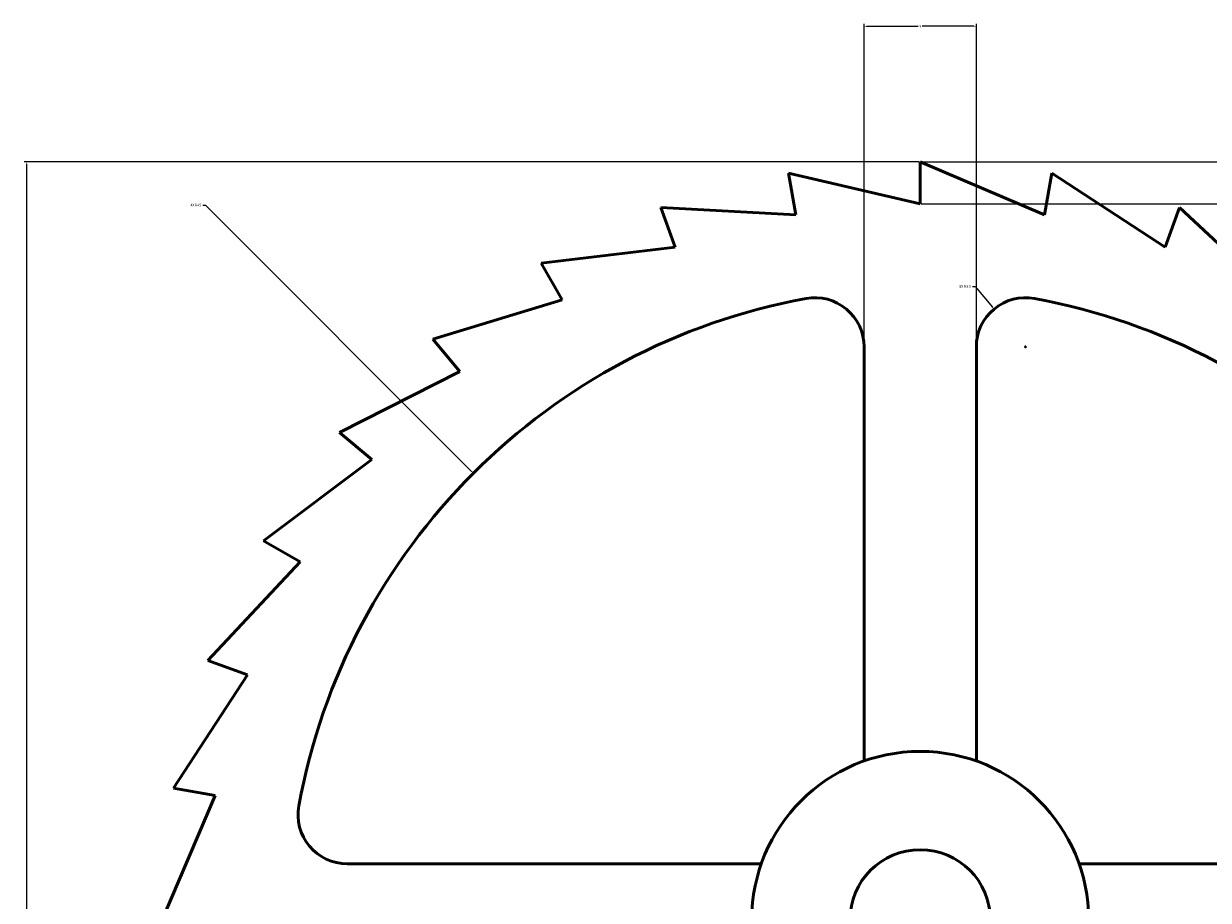
# Model space of a CAD drawing. Units: millimetres. Extents: x 3287 to 3415, y 1573 to 1701.
# Tile 2 of 3: x 3287 to 3371, y 1639 to 1701. Entities that reach past the tile are written whole.
import ezdxf

# ---------------------------------------------------------------- set-up
doc = ezdxf.new("R2010")
doc.units = ezdxf.units.MM
doc.layers.add('M-DIMS', color=2, linetype='Continuous', lineweight=18)
doc.layers.add('M-OUTL', color=7, linetype='Continuous', lineweight=50)
doc.styles.get("Standard").update_dxf_attribs({"font": 'arial.ttf'})
doc.dimstyles.get("Standard").update_dxf_attribs({"dimtxt": 0.18, "dimasz": 0.18, "dimexe": 0.18, "dimexo": 0.0625, "dimgap": 0.09, "dimtad": 0, "dimtih": 1, "dimtoh": 1, "dimdec": 4, "dimzin": 0, "dimdsep": 46, "dimtxsty": 'Standard', "dimcen": 0.09, "dimadec": 0, "dimazin": 0, "dimtfac": 1, "dimtdec": 4, "dimtofl": 0, "dimtmove": 0, "dimatfit": 3, "dimfxl": 1, "dimtolj": 1, "dimtzin": 0, "dimarcsym": 0})

# ---------------------------------------------------------------- blocks, each defined once
blk = doc.blocks.new('RATCHET-TOOTH-10DEG')
for p, q in [((0, 8.856), (2.954, 9.377)), ((2.954, 9.377), (0.775, 0))]:
    blk.add_line(p, q)
blk = doc.blocks.new('WHEEL-SPOKE-OPENING')
for points in [[(40.317, 7.314), (40.317, 36.817)], [(3.5, 0), (33.003, 0)]]:
    blk.add_lwpolyline(points)
for centre, radius, start, end in [((44.317, -4), 45, 100.41187, 169.58813), ((36.817, 36.817), 3.5, 0, 100.41187), ((3.5, 3.5), 3.5, 169.58813, 270)]:
    blk.add_arc(centre, radius, start, end)
blk = doc.blocks.new('*D4')
at = {"layer": 'Defpoints', "color": 0, "transparency": 16777216}
for p in [(3287.322, 1691.286), (3350.972, 1691.286), (3350.972, 1583.286)]:
    blk.add_point(p, dxfattribs=at)
at = {"layer": 'M-DIMS', "color": 0, "lineweight": -2, "transparency": 16777216}
for p, q in [((3350.909, 1691.286), (3287.142, 1691.286)), ((3287.322, 1691.106), (3287.322, 1637.468)), ((3287.322, 1583.466), (3287.322, 1637.104)), ((3350.909, 1583.286), (3287.142, 1583.286))]:
    blk.add_line(p, q, dxfattribs=at)
at = {"layer": 'M-DIMS', "color": 0, "transparency": 16777216}
for points in [[(3287.292, 1691.106), (3287.352, 1691.106), (3287.322, 1691.286)], [(3287.292, 1583.466), (3287.352, 1583.466), (3287.322, 1583.286)]]:
    blk.add_solid(points, dxfattribs=at)
at = {"layer": 'M-DIMS', "color": 0, "transparency": 16777216, "insert": (3287.322, 1637.286), "char_height": 0.18, "attachment_point": 5}
blk.add_mtext('\\A1;108', dxfattribs=at)
blk = doc.blocks.new('*D5')
at = {"layer": 'Defpoints', "color": 0, "transparency": 16777216}
for p in [(3350.972, 1691.286), (3350.972, 1688.286), (3414.622, 1688.286)]:
    blk.add_point(p, dxfattribs=at)
at = {"layer": 'M-DIMS', "color": 0, "lineweight": -2, "transparency": 16777216}
for p, q in [((3351.034, 1691.286), (3414.802, 1691.286)), ((3414.622, 1691.106), (3414.622, 1689.968)), ((3414.622, 1688.466), (3414.622, 1689.604)), ((3351.034, 1688.286), (3414.802, 1688.286))]:
    blk.add_line(p, q, dxfattribs=at)
at = {"layer": 'M-DIMS', "color": 0, "transparency": 16777216}
for points in [[(3414.592, 1691.106), (3414.652, 1691.106), (3414.622, 1691.286)], [(3414.592, 1688.466), (3414.652, 1688.466), (3414.622, 1688.286)]]:
    blk.add_solid(points, dxfattribs=at)
at = {"layer": 'M-DIMS', "color": 0, "transparency": 16777216, "insert": (3414.622, 1689.786), "char_height": 0.18, "attachment_point": 5}
blk.add_mtext('\\A1;3', dxfattribs=at)
blk = doc.blocks.new('*D6')
at = {"layer": 'Defpoints', "color": 0, "transparency": 16777216}
for p in [(3354.972, 1700.936), (3346.972, 1678.103), (3354.972, 1678.103)]:
    blk.add_point(p, dxfattribs=at)
at = {"layer": 'M-DIMS', "color": 0, "lineweight": -2, "transparency": 16777216}
for p, q in [((3346.972, 1678.165), (3346.972, 1701.116)), ((3354.972, 1678.165), (3354.972, 1701.116)), ((3347.152, 1700.936), (3350.822, 1700.936)), ((3354.792, 1700.936), (3351.121, 1700.936))]:
    blk.add_line(p, q, dxfattribs=at)
at = {"layer": 'M-DIMS', "color": 0, "transparency": 16777216}
for points in [[(3347.152, 1700.966), (3347.152, 1700.906), (3346.972, 1700.936)], [(3354.792, 1700.966), (3354.792, 1700.906), (3354.972, 1700.936)]]:
    blk.add_solid(points, dxfattribs=at)
at = {"layer": 'M-DIMS', "color": 0, "transparency": 16777216, "insert": (3350.972, 1700.936), "char_height": 0.18, "attachment_point": 5}
blk.add_mtext('\\A1;8', dxfattribs=at)
blk = doc.blocks.new('*D7')
at = {"layer": 'Defpoints', "color": 0, "transparency": 16777216}
for p in [(3319.152, 1669.106), (3350.972, 1637.286)]:
    blk.add_point(p, dxfattribs=at)
at = {"layer": 'M-DIMS', "color": 0, "lineweight": -2, "transparency": 16777216}
for p, q in [((3299.88, 1688.198), (3300.06, 1688.198)), ((3300.06, 1688.198), (3319.025, 1669.233)), ((3350.882, 1637.286), (3351.062, 1637.286)), ((3350.972, 1637.196), (3350.972, 1637.376))]:
    blk.add_line(p, q, dxfattribs=at)
at = {"layer": 'M-DIMS', "color": 0, "transparency": 16777216}
blk.add_solid([(3319.046, 1669.254), (3319.004, 1669.212), (3319.152, 1669.106)], dxfattribs=at)
at = {"layer": 'M-DIMS', "color": 0, "transparency": 16777216, "insert": (3299.377, 1688.198), "char_height": 0.18, "attachment_point": 5}
blk.add_mtext('\\A1;4X R45', dxfattribs=at)
blk = doc.blocks.new('*D8')
at = {"layer": 'Defpoints', "color": 0, "transparency": 16777216}
for p in [(3356.232, 1680.792), (3358.472, 1678.103)]:
    blk.add_point(p, dxfattribs=at)
at = {"layer": 'M-DIMS', "color": 0, "lineweight": -2, "transparency": 16777216}
for p, q in [((3354.708, 1682.406), (3354.888, 1682.406)), ((3354.888, 1682.406), (3356.117, 1680.931)), ((3358.382, 1678.103), (3358.562, 1678.103)), ((3358.472, 1678.013), (3358.472, 1678.193))]:
    blk.add_line(p, q, dxfattribs=at)
at = {"layer": 'M-DIMS', "color": 0, "transparency": 16777216}
blk.add_solid([(3356.14, 1680.95), (3356.094, 1680.911), (3356.232, 1680.792)], dxfattribs=at)
at = {"layer": 'M-DIMS', "color": 0, "transparency": 16777216, "insert": (3354.174, 1682.406), "char_height": 0.18, "attachment_point": 5}
blk.add_mtext('\\A1;8X R3.5', dxfattribs=at)

msp = doc.modelspace()

# ---------------------------------------------------------------- linework, layer by layer
at = {"layer": 'M-OUTL'}
for radius in [12, 5]:
    msp.add_circle((3350.972, 1637.286), radius, dxfattribs=at)

# ---------------------------------------------------------------- block references
for name, p, rotation in [('RATCHET-TOOTH-10DEG', (3359.693, 1686.748), 79.99999999999987), ('RATCHET-TOOTH-10DEG', (3350.972, 1687.511), 90.00000000000333), ('RATCHET-TOOTH-10DEG', (3368.15, 1684.482), 69.99999999999669), ('RATCHET-TOOTH-10DEG', (3342.25, 1686.748), 100.0000000000026), ('RATCHET-TOOTH-10DEG', (3376.084, 1680.782), 60.00000000000543), ('RATCHET-TOOTH-10DEG', (3333.794, 1684.482), 109.9999999999977), ('RATCHET-TOOTH-10DEG', (3325.859, 1680.783), 119.9999999999948), ('WHEEL-SPOKE-OPENING', (3354.972, 1681.603), 270.0000000000003), ('RATCHET-TOOTH-10DEG', (3318.688, 1675.761), 129.9999999999969), ('RATCHET-TOOTH-10DEG', (3312.497, 1669.57), 140.0000000000046), ('RATCHET-TOOTH-10DEG', (3307.475, 1662.399), 150.0000000000002), ('RATCHET-TOOTH-10DEG', (3303.775, 1654.464), 160.0000000000042), ('RATCHET-TOOTH-10DEG', (3301.509, 1646.008), 169.9999999999888)]:
    msp.add_blockref(name, p, dxfattribs=dict(at, rotation=rotation))
msp.add_blockref('WHEEL-SPOKE-OPENING', (3306.655, 1641.286), dxfattribs=at)

# ---------------------------------------------------------------- dimensions: what is measured, and where the dimension line sits
at = {"layer": 'M-DIMS'}
dim = msp.add_linear_dim(base=(3354.972, 1700.936), p1=(3346.972, 1678.103), p2=(3354.972, 1678.103), dimstyle='Standard', override={"dimdec": 0, "dimlfac": 1, "dimrnd": 0, "dimzin": 0, "dimdsep": 46, "dimlunit": 2}, dxfattribs=at)
dim.commit()
dim.dimension.update_dxf_attribs({"geometry": '*D6', "text_midpoint": (3350.972, 1700.936)})
for base, p1, p2, picture, middle in [((3287.322, 1691.286), (3350.972, 1583.286), (3350.972, 1691.286), '*D4', (3287.322, 1637.286)), ((3414.622, 1688.286), (3350.972, 1691.286), (3350.972, 1688.286), '*D5', (3414.622, 1689.786))]:
    dim = msp.add_linear_dim(base=base, p1=p1, p2=p2, angle=90, dimstyle='Standard', override={"dimdec": 0, "dimlfac": 1, "dimrnd": 0, "dimzin": 0, "dimdsep": 46, "dimlunit": 2}, dxfattribs=at)
    dim.commit()
    dim.dimension.update_dxf_attribs({"geometry": picture, "text_midpoint": middle})
for center, mpoint, text, override, picture, middle in [((3350.972, 1637.286), (3319.152, 1669.106), '4X <>', {"dimdec": 0, "dimlfac": 1, "dimrnd": 0, "dimzin": 0, "dimdsep": 46, "dimlunit": 2}, '*D7', (3299.377, 1688.198)), ((3358.472, 1678.103), (3356.232, 1680.792), '8X <>', {"dimdec": 1, "dimlfac": 1, "dimrnd": 0, "dimzin": 0, "dimdsep": 46, "dimlunit": 2}, '*D8', (3354.174, 1682.406))]:
    dim = msp.add_radius_dim(center=center, mpoint=mpoint, text=text, dimstyle='Standard', override=override, dxfattribs=at)
    dim.commit()
    dim.dimension.update_dxf_attribs({"geometry": picture, "text_midpoint": middle, "dimtype": 164})

doc.saveas('drawing.dxf')
